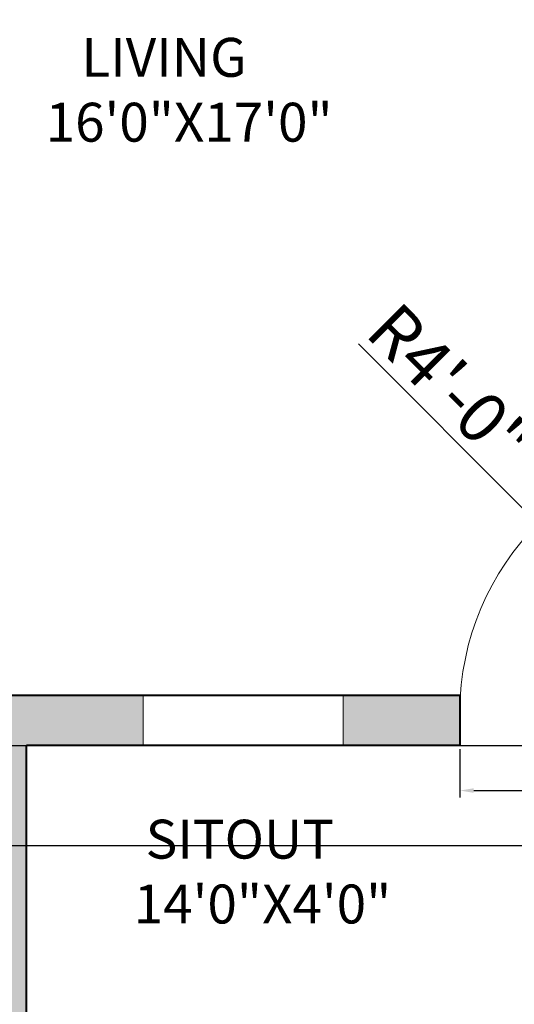
# Model space of a CAD drawing. Units: inches. Extents: x 2337 to 3570, y 1258 to 1938.
# Tile 22 of 30: x 3293 to 3382, y 1496 to 1673. Entities that reach past the tile are written whole.
import ezdxf

# ---------------------------------------------------------------- set-up
doc = ezdxf.new("R2010")
doc.units = ezdxf.units.IN
for name, color, linetype, lineweight in [('A-ANNO-DIMS', 2, 'Continuous', 18), ('A-AREA-IDEN', 7, 'Continuous', 18), ('A-DOOR', 4, 'Continuous', 20), ('A-GLAZ', 4, 'Continuous', 18), ('A-WALL', 7, 'Continuous', 40)]:
    doc.layers.add(name, color=color, linetype=linetype, lineweight=lineweight)
doc.layers.add('A-WALL-PATT', color=18, linetype='Continuous', lineweight=13, true_color=0x000000)
doc.styles.get("Standard").update_dxf_attribs({"font": 'arial.ttf'})
doc.dimstyles.new('ISO-25', dxfattribs={"dimtxt": 9, "dimasz": 2.5, "dimexe": 1.25, "dimexo": 0.625, "dimtad": 1, "dimdec": 1, "dimlunit": 3, "dimtxsty": 'Standard', "dimcen": 2.5, "dimadec": 0, "dimazin": 0, "dimtfac": 1, "dimtdec": 1, "dimtmove": 0, "dimatfit": 3, "dimfxl": 1, "dimarcsym": 0})

# ---------------------------------------------------------------- blocks, each defined once
blk = doc.blocks.new('DOOR-SWING-48IN')
for p, q in [((0, 6), (0, 0)), ((48, 6), (48, 0))]:
    blk.add_line(p, q)
blk.add_lwpolyline([(48, 6), (48, 54), (46.25, 54), (46.25, 6)], close=True)
blk.add_arc((48, 6), 48, 90, 180)
blk = doc.blocks.new('*D69')
at = {"layer": 'A-ANNO-DIMS', "color": 0, "lineweight": -2, "transparency": 16777216}
for p, q in [((3371.79, 1541.49), (3371.79, 1532.77)), ((3419.79, 1541.49), (3419.79, 1532.77)), ((3374.29, 1534.02), (3417.29, 1534.02)), ((3419.79, 1534.02), (3478.76, 1534.02))]:
    blk.add_line(p, q, dxfattribs=at)
at = {"layer": 'A-ANNO-DIMS', "color": 0, "transparency": 16777216}
for points in [[(3374.29, 1534.43), (3374.29, 1533.6), (3371.79, 1534.02)], [(3417.29, 1534.43), (3417.29, 1533.6), (3419.79, 1534.02)]]:
    blk.add_solid(points, dxfattribs=at)
at = {"layer": 'Defpoints', "color": 0, "transparency": 16777216}
for p in [(3371.79, 1542.12), (3419.79, 1542.12), (3419.79, 1534.02)]:
    blk.add_point(p, dxfattribs=at)
at = {"layer": 'A-ANNO-DIMS', "color": 0, "transparency": 16777216, "insert": (3450.52, 1539.24), "char_height": 9, "attachment_point": 5}
blk.add_mtext('4\'-0" TYP.', dxfattribs=at)
blk = doc.blocks.new('*D115')
at = {"layer": 'A-ANNO-DIMS', "color": 0, "lineweight": -2, "transparency": 16777216}
for p, q in [((3243.41, 1542.12), (3502.44, 1542.12)), ((3501.19, 1539.62), (3501.19, 1526.62)), ((3243.41, 1524.12), (3502.44, 1524.12)), ((3501.19, 1524.12), (3501.19, 1497.29))]:
    blk.add_line(p, q, dxfattribs=at)
at = {"layer": 'A-ANNO-DIMS', "color": 0, "transparency": 16777216}
for points in [[(3500.77, 1539.62), (3501.6, 1539.62), (3501.19, 1542.12)], [(3500.77, 1526.62), (3501.6, 1526.62), (3501.19, 1524.12)]]:
    blk.add_solid(points, dxfattribs=at)
at = {"layer": 'Defpoints', "color": 0, "transparency": 16777216}
for p in [(3242.79, 1542.12), (3242.79, 1524.12), (3501.19, 1524.12)]:
    blk.add_point(p, dxfattribs=at)
at = {"layer": 'A-ANNO-DIMS', "color": 0, "transparency": 16777216, "insert": (3495.97, 1509.45), "char_height": 9, "attachment_point": 5, "rotation": 90}
blk.add_mtext('1\'-6"', dxfattribs=at)
blk = doc.blocks.new('*D120')
at = {"layer": 'A-ANNO-DIMS', "color": 0, "lineweight": -2, "transparency": 16777216}
for p, q in [((3353.53, 1614.37), (3384.08, 1583.82)), ((3419.79, 1548.12), (3385.84, 1582.06))]:
    blk.add_line(p, q, dxfattribs=at)
at = {"layer": 'A-ANNO-DIMS', "color": 0, "transparency": 16777216}
blk.add_solid([(3384.37, 1584.12), (3383.78, 1583.53), (3385.84, 1582.06)], dxfattribs=at)
at = {"layer": 'Defpoints', "color": 0, "transparency": 16777216}
for p in [(3385.84, 1582.06), (3419.79, 1548.12)]:
    blk.add_point(p, dxfattribs=at)
at = {"layer": 'A-ANNO-DIMS', "color": 0, "transparency": 16777216, "insert": (3369.17, 1606.11), "char_height": 9, "attachment_point": 5, "rotation": 315.0001}
blk.add_mtext('R4\'-0"', dxfattribs=at)

msp = doc.modelspace()

# ---------------------------------------------------------------- hatches: boundary and pattern name
at = {"layer": 'A-WALL-PATT'}
h = msp.add_hatch(color=256, dxfattribs=at)
h.dxf.hatch_style = 1
h.paths.add_polyline_path([(3233.79, 1857.12), (3017.79, 1857.12), (3017.79, 1824.12), (3026.79, 1824.12), (3026.79, 1848.12), (3233.79, 1848.12)])
h.paths.add_polyline_path([(3128.79, 1764.12), (3026.79, 1764.12), (3026.79, 1788.12), (3017.79, 1788.12), (3017.79, 1743.12), (3026.79, 1743.12), (3026.79, 1755.12), (3128.79, 1755.12)])
h.paths.add_polyline_path([(3245.79, 1761.12), (3245.79, 1764.12), (3164.79, 1764.12), (3164.79, 1755.12), (3170.79, 1755.12), (3170.79, 1701.12), (3224.79, 1701.12), (3224.79, 1605.12), (3233.79, 1605.12), (3233.79, 1713.12), (3224.79, 1713.12), (3224.79, 1707.12), (3176.79, 1707.12), (3176.79, 1755.12), (3224.79, 1755.12), (3224.79, 1749.12), (3233.79, 1749.12), (3233.79, 1755.12), (3245.79, 1755.12)])
h.paths.add_polyline_path([(3026.79, 1707.12), (3017.79, 1707.12), (3017.79, 1617.12), (3026.79, 1617.12), (3026.79, 1635.12), (3068.79, 1635.12), (3068.79, 1641.12), (3026.79, 1641.12)])
h.paths.add_polyline_path([(3104.79, 1551.12), (3026.79, 1551.12), (3026.79, 1569.12), (3017.79, 1569.12), (3017.79, 1518.12), (3026.79, 1518.12), (3026.79, 1542.12), (3104.79, 1542.12)])
h.paths.add_polyline_path([(3026.79, 1482.12), (3017.79, 1482.12), (3017.79, 1410.12), (3026.79, 1410.12)])
h.paths.add_polyline_path([(3188.79, 1350.12), (3152.79, 1350.12), (3152.79, 1380.12), (3146.79, 1380.12), (3146.79, 1350.12), (3026.79, 1350.12), (3026.79, 1374.12), (3017.79, 1374.12), (3017.79, 1341.12), (3188.79, 1341.12)])
h.paths.add_polyline_path([(3224.79, 1416.12), (3248.79, 1416.12), (3248.79, 1422.12), (3152.79, 1422.12), (3152.79, 1542.12), (3242.79, 1542.12), (3242.79, 1551.12), (3233.79, 1551.12), (3233.79, 1557.12), (3224.79, 1557.12), (3224.79, 1551.12), (3140.79, 1551.12), (3140.79, 1542.12), (3146.79, 1542.12), (3146.79, 1410.12), (3152.79, 1410.12), (3152.79, 1416.12), (3218.79, 1416.12), (3218.79, 1350.12), (3212.79, 1350.12), (3212.79, 1341.12), (3293.79, 1341.12), (3293.79, 1362.12), (3284.79, 1362.12), (3284.79, 1350.12), (3224.79, 1350.12)])
h.paths.add_polyline_path([(3293.79, 1434.12), (3284.79, 1434.12), (3284.79, 1422.12), (3278.79, 1422.12), (3278.79, 1416.12), (3284.79, 1416.12), (3284.79, 1386.12), (3293.79, 1386.12)], flags=17)
h.paths.add_polyline_path([(3293.79, 1542.12), (3314.79, 1542.12), (3314.79, 1551.12), (3278.79, 1551.12), (3278.79, 1545.12), (3278.79, 1542.12), (3284.79, 1542.12), (3284.79, 1482.12), (3293.79, 1482.12)])
h.paths.add_polyline_path([(3371.79, 1551.12), (3350.79, 1551.12), (3350.79, 1542.12), (3371.79, 1542.12), (3371.79, 1548.12)])
h.paths.add_polyline_path([(3434.79, 1647.12), (3425.79, 1647.12), (3425.79, 1551.12), (3419.79, 1551.12), (3419.79, 1548.12), (3419.79, 1542.12), (3434.79, 1542.12)])
h.paths.add_polyline_path([(3434.79, 1764.12), (3389.79, 1764.12), (3389.79, 1755.12), (3425.79, 1755.12), (3425.79, 1719.12), (3434.79, 1719.12)])
h.paths.add_polyline_path([(3317.79, 1764.12), (3281.79, 1764.12), (3281.79, 1755.12), (3317.79, 1755.12)])

# ---------------------------------------------------------------- linework, layer by layer
at = {"layer": 'A-GLAZ'}
for p, q in [((3314.79, 1542.12), (3314.79, 1551.12)), ((3350.79, 1542.12), (3350.79, 1551.12))]:
    msp.add_line(p, q, dxfattribs=at)
at = {"layer": 'A-WALL'}
for p, q in [((3371.79, 1551.12), (3278.79, 1551.12)), ((3371.79, 1551.12), (3371.79, 1542.12)), ((3293.79, 1341.12), (3293.79, 1542.12)), ((3371.79, 1542.12), (3293.79, 1542.12))]:
    msp.add_line(p, q, dxfattribs=at)

# ---------------------------------------------------------------- block references
at = {"layer": 'A-DOOR'}
msp.add_blockref('DOOR-SWING-48IN', (3371.79, 1542.12), dxfattribs=at)

# ---------------------------------------------------------------- texts
at = {"layer": 'A-AREA-IDEN', "char_height": 7, "attachment_point": 1}
for s, insert in [('   LIVING\\P16\'0"X17\'0"', (3297.26, 1669.44)), (' SITOUT\\P14\'0"X4\'0"', (3313.11, 1528.77))]:
    msp.add_mtext_dynamic_manual_height_columns(s, width=66.911, gutter_width=12.5, heights=[0], dxfattribs=dict(at, insert=insert))

# ---------------------------------------------------------------- dimensions: what is measured, and where the dimension line sits
at = {"layer": 'A-ANNO-DIMS'}
dim = msp.add_radius_dim(center=(3419.79, 1548.12), mpoint=(3385.84, 1582.06), dimstyle='ISO-25', override={"dimdec": 1, "dimlfac": 1, "dimrnd": 0, "dimzin": 1, "dimdsep": 46, "dimlunit": 4, "dimfrac": 2}, dxfattribs=at)
dim.commit()
dim.dimension.update_dxf_attribs({"geometry": '*D120', "text_midpoint": (3365.48, 1602.42), "dimtype": 164})
dim = msp.add_linear_dim(base=(3419.79, 1534.02), p1=(3371.79, 1542.12), p2=(3419.79, 1542.12), text='<> TYP.', dimstyle='ISO-25', override={"dimdec": 1, "dimlfac": 1, "dimrnd": 0, "dimzin": 1, "dimdsep": 46, "dimlunit": 4, "dimfrac": 2}, dxfattribs=at)
dim.commit()
dim.dimension.update_dxf_attribs({"geometry": '*D69', "text_midpoint": (3450.52, 1539.24)})
dim = msp.add_linear_dim(base=(3501.19, 1524.12), p1=(3242.79, 1542.12), p2=(3242.79, 1524.12), angle=90, dimstyle='ISO-25', override={"dimdec": 1, "dimlfac": 1, "dimrnd": 0, "dimzin": 1, "dimdsep": 46, "dimlunit": 4, "dimfrac": 2}, dxfattribs=at)
dim.commit()
dim.dimension.update_dxf_attribs({"geometry": '*D115', "text_midpoint": (3495.97, 1509.45)})

doc.saveas('drawing.dxf')
